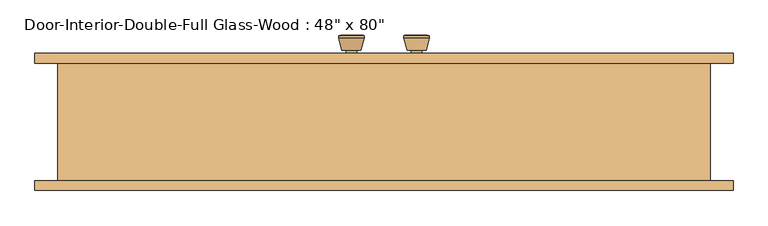
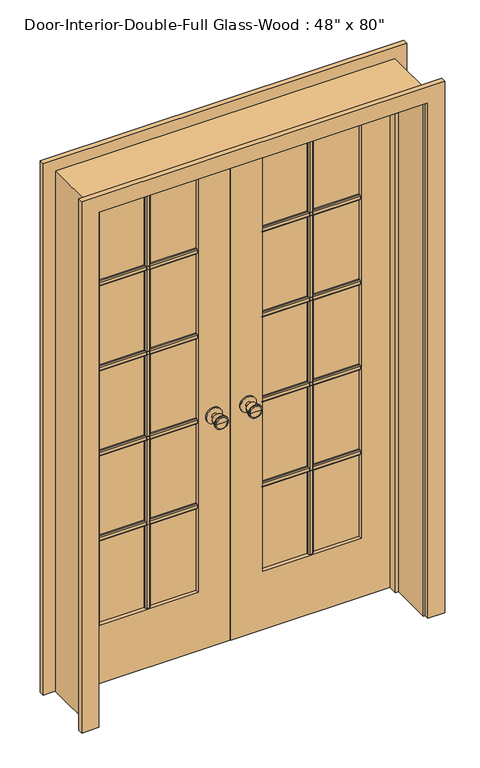
"""IFC4 building model written with IfcOpenShell, lengths in millimetres: door geometry."""

from ifc_helpers import new_model, si_unit, point, frame, frame_2d, origin, place, context, project, spatial, polyline, circle_curve, trimmed, segment, composite_curve, outline, extrude, faceted_brep, source, transform, mapped, element, save
from ifc_brep_helpers import plane_surface, cylinder_surface, revolved_surface, advanced_brep


def door_cd3c5da8(model_context):
    return source(origin(), model_context, "Body", "SolidModel", [
        advanced_brep(
        [(-63.5, 117.125, 914.4), (-73.5, 117.125, 914.4), (-53.5, 117.125, 914.4), (-83.9758676, 166.125, 914.4), (-63.5, 166.125, 914.4), (-43.0241324, 166.125, 914.4), (-88.5, 164.2971319, 914.4), (-38.5, 164.2971319, 914.4), (-88.5, 160.8334537, 914.4), (-38.5, 160.8334537, 914.4), (-82.136236, 136.125, 914.4), (-44.863764, 136.125, 914.4), (-73.5, 136.125, 914.4), (-53.5, 136.125, 914.4)],
        [
            (0, 1),
            (1, 2, circle_curve(frame((-63.5, 117.125, 914.4), z_axis=(0.0, -1.0, 0.0), x_axis=(1.0, 0.0, 0.0)), 10.0)),
            (2, 0),
            (2, 1, circle_curve(frame((-63.5, 117.125, 914.4), z_axis=(0.0, -1.0, 0.0), x_axis=(1.0, 0.0, 0.0)), 10.0)),
            (3, 4),
            (4, 5),
            (5, 3, circle_curve(frame((-63.5, 166.125, 914.4), z_axis=(0.0, 1.0, 0.0), x_axis=(1.0, 0.0, 0.0)), 20.4758676)),
            (3, 5, circle_curve(frame((-63.5, 166.125, 914.4), z_axis=(0.0, 1.0, 0.0), x_axis=(1.0, 0.0, 0.0)), 20.4758676)),
            (6, 3),
            (5, 7),
            (7, 6, circle_curve(frame((-63.5, 164.2971319, 914.4), z_axis=(0.0, 1.0, 0.0), x_axis=(1.0, 0.0, 0.0)), 25.0)),
            (6, 7, circle_curve(frame((-63.5, 164.2971319, 914.4), z_axis=(0.0, 1.0, 0.0), x_axis=(1.0, 0.0, 0.0)), 25.0)),
            (8, 6),
            (7, 9),
            (9, 8, circle_curve(frame((-63.5, 160.8334537, 914.4), z_axis=(0.0, 1.0, 0.0), x_axis=(1.0, 0.0, 0.0)), 25.0)),
            (8, 9, circle_curve(frame((-63.5, 160.8334537, 914.4), z_axis=(0.0, 1.0, 0.0), x_axis=(1.0, 0.0, 0.0)), 25.0)),
            (10, 8),
            (9, 11),
            (11, 10, circle_curve(frame((-63.5, 136.125, 914.4), z_axis=(0.0, 1.0, 0.0), x_axis=(1.0, 0.0, 0.0)), 18.636236)),
            (10, 11, circle_curve(frame((-63.5, 136.125, 914.4), z_axis=(0.0, 1.0, 0.0), x_axis=(1.0, 0.0, 0.0)), 18.636236)),
            (12, 10),
            (11, 13),
            (13, 12, circle_curve(frame((-63.5, 136.125, 914.4), z_axis=(0.0, 1.0, 0.0), x_axis=(1.0, 0.0, 0.0)), 10.0)),
            (12, 13, circle_curve(frame((-63.5, 136.125, 914.4), z_axis=(0.0, 1.0, 0.0), x_axis=(1.0, 0.0, 0.0)), 10.0)),
            (1, 12),
            (13, 2),
        ],
        [
            plane_surface(frame((-63.5, 117.125, 914.4), z_axis=(0.0, -1.0, 0.0), x_axis=(1.0, 0.0, 0.0))),
            plane_surface(frame((-63.5, 166.125, 914.4), z_axis=(0.0, 1.0, 0.0), x_axis=(1.0, 0.0, 0.0))),
            revolved_surface(polyline([(-43.0241324, 166.125, 914.4), (-38.5, 164.2971319, 914.4)]), (-63.5, 117.125, 914.4), (0.0, -1.0, 0.0)),
            cylinder_surface(frame((-63.5, 117.125, 914.4), z_axis=(0.0, -1.0, 0.0), x_axis=(1.0, 0.0, 0.0)), 25.0),
            revolved_surface(polyline([(-38.5, 160.8334537, 914.4), (-44.863764, 136.125, 914.4)]), (-63.5, 117.125, 914.4), (0.0, -1.0, 0.0)),
            plane_surface(frame((-63.5, 136.125, 914.4), z_axis=(0.0, -1.0, 0.0), x_axis=(1.0, 0.0, 0.0))),
            cylinder_surface(frame((-63.5, 117.125, 914.4), z_axis=(0.0, -1.0, 0.0), x_axis=(1.0, 0.0, 0.0)), 10.0),
        ],
        [
            (0, [[1, 2, 3]]),
            (0, [[-3, 4, -1]]),
            (1, [[5, 6, 7]]),
            (1, [[-6, -5, 8]]),
            (2, [[9, -7, 10, 11]]),
            (2, [[-10, -8, -9, 12]]),
            (3, [[13, -11, 14, 15]]),
            (3, [[-14, -12, -13, 16]]),
            (4, [[17, -15, 18, 19]]),
            (4, [[-18, -16, -17, 20]]),
            (5, [[21, -19, 22, 23]]),
            (5, [[-22, -20, -21, 24]]),
            (6, [[25, -23, 26, -2]]),
            (6, [[-26, -24, -25, -4]]),
        ],
    ),
        extrude(outline(composite_curve([segment(trimmed(circle_curve(frame_2d((914.4, -63.5)), 30.0), [point((914.4, -33.5))], [point((914.4, -93.5))], False, "CARTESIAN"), True, "CONTINUOUS"), segment(trimmed(circle_curve(frame_2d((914.4, -63.5)), 30.0), [point((914.4, -93.5))], [point((914.4, -33.5))], False, "CARTESIAN"), True, "CONTINUOUS")], self_intersect=False)), frame((0.0, 111.125, 0.0), z_axis=(0.0, 1.0, 0.0), x_axis=(0.0, 0.0, 1.0)), (0.0, 0.0, 1.0), 6.0),
        advanced_brep(
        [(-63.5, 70.2, 914.4), (-53.5, 70.2, 914.4), (-73.5, 70.2, 914.4), (-83.9758676, 21.2, 914.4), (-43.0241324, 21.2, 914.4), (-63.5, 21.2, 914.4), (-88.5, 23.0278681, 914.4), (-38.5, 23.0278681, 914.4), (-88.5, 26.4915463, 914.4), (-38.5, 26.4915463, 914.4), (-82.136236, 51.2, 914.4), (-44.863764, 51.2, 914.4), (-73.5, 51.2, 914.4), (-53.5, 51.2, 914.4)],
        [
            (0, 1),
            (1, 2, circle_curve(frame((-63.5, 70.2, 914.4), z_axis=(0.0, 1.0, 0.0), x_axis=(1.0, 0.0, 0.0)), 10.0)),
            (2, 0),
            (2, 1, circle_curve(frame((-63.5, 70.2, 914.4), z_axis=(0.0, 1.0, 0.0), x_axis=(1.0, 0.0, 0.0)), 10.0)),
            (3, 4, circle_curve(frame((-63.5, 21.2, 914.4), z_axis=(0.0, -1.0, 0.0), x_axis=(1.0, 0.0, 0.0)), 20.4758676)),
            (4, 5),
            (5, 3),
            (4, 3, circle_curve(frame((-63.5, 21.2, 914.4), z_axis=(0.0, -1.0, 0.0), x_axis=(1.0, 0.0, 0.0)), 20.4758676)),
            (6, 7, circle_curve(frame((-63.5, 23.0278681, 914.4), z_axis=(0.0, -1.0, 0.0), x_axis=(1.0, 0.0, 0.0)), 25.0)),
            (7, 4),
            (3, 6),
            (7, 6, circle_curve(frame((-63.5, 23.0278681, 914.4), z_axis=(0.0, -1.0, 0.0), x_axis=(1.0, 0.0, 0.0)), 25.0)),
            (8, 9, circle_curve(frame((-63.5, 26.4915463, 914.4), z_axis=(0.0, -1.0, 0.0), x_axis=(1.0, 0.0, 0.0)), 25.0)),
            (9, 7),
            (6, 8),
            (9, 8, circle_curve(frame((-63.5, 26.4915463, 914.4), z_axis=(0.0, -1.0, 0.0), x_axis=(1.0, 0.0, 0.0)), 25.0)),
            (10, 11, circle_curve(frame((-63.5, 51.2, 914.4), z_axis=(0.0, -1.0, 0.0), x_axis=(1.0, 0.0, 0.0)), 18.636236)),
            (11, 9),
            (8, 10),
            (11, 10, circle_curve(frame((-63.5, 51.2, 914.4), z_axis=(0.0, -1.0, 0.0), x_axis=(1.0, 0.0, 0.0)), 18.636236)),
            (12, 13, circle_curve(frame((-63.5, 51.2, 914.4), z_axis=(0.0, -1.0, 0.0), x_axis=(1.0, 0.0, 0.0)), 10.0)),
            (13, 11),
            (10, 12),
            (13, 12, circle_curve(frame((-63.5, 51.2, 914.4), z_axis=(0.0, -1.0, 0.0), x_axis=(1.0, 0.0, 0.0)), 10.0)),
            (1, 13),
            (12, 2),
        ],
        [
            plane_surface(frame((-63.5, 70.2, 914.4), z_axis=(0.0, 1.0, 0.0), x_axis=(1.0, 0.0, 0.0))),
            plane_surface(frame((-63.5, 21.2, 914.4), z_axis=(0.0, -1.0, 0.0), x_axis=(1.0, 0.0, 0.0))),
            revolved_surface(polyline([(-43.0241324, 21.2, 914.4), (-38.5, 23.0278681, 914.4)]), (-63.5, 70.2, 914.4), (0.0, 1.0, 0.0)),
            cylinder_surface(frame((-63.5, 70.2, 914.4), z_axis=(0.0, 1.0, 0.0), x_axis=(1.0, 0.0, 0.0)), 25.0),
            revolved_surface(polyline([(-38.5, 26.4915463, 914.4), (-44.863764, 51.2, 914.4)]), (-63.5, 70.2, 914.4), (0.0, 1.0, 0.0)),
            plane_surface(frame((-63.5, 51.2, 914.4), z_axis=(0.0, 1.0, 0.0), x_axis=(1.0, 0.0, 0.0))),
            cylinder_surface(frame((-63.5, 70.2, 914.4), z_axis=(0.0, 1.0, 0.0), x_axis=(1.0, 0.0, 0.0)), 10.0),
        ],
        [
            (0, [[1, 2, 3]]),
            (0, [[-3, 4, -1]]),
            (1, [[5, 6, 7]]),
            (1, [[8, -7, -6]]),
            (2, [[9, 10, -5, 11]]),
            (2, [[12, -11, -8, -10]]),
            (3, [[13, 14, -9, 15]]),
            (3, [[16, -15, -12, -14]]),
            (4, [[17, 18, -13, 19]]),
            (4, [[20, -19, -16, -18]]),
            (5, [[21, 22, -17, 23]]),
            (5, [[24, -23, -20, -22]]),
            (6, [[-2, 25, -21, 26]]),
            (6, [[-4, -26, -24, -25]]),
        ],
    ),
        extrude(outline(composite_curve([segment(trimmed(circle_curve(frame_2d((914.4, -63.5)), 30.0), [point((914.4, -33.5))], [point((914.4, -93.5))], False, "CARTESIAN"), True, "CONTINUOUS"), segment(trimmed(circle_curve(frame_2d((914.4, -63.5)), 30.0), [point((914.4, -93.5))], [point((914.4, -33.5))], False, "CARTESIAN"), True, "CONTINUOUS")], self_intersect=False)), frame((0.0, 70.2, 0.0), z_axis=(0.0, 1.0, 0.0), x_axis=(0.0, 0.0, 1.0)), (0.0, 0.0, 1.0), 6.0),
        extrude(outline(polyline([(90.17, 1586.23), (90.17, 1567.18), (83.82, 1567.18), (80.645, 1570.355), (80.645, 1583.055), (83.82, 1586.23), (90.17, 1586.23)])), frame((120.65, 0.0, 0.0), z_axis=(1.0, 0.0, 0.0), x_axis=(0.0, 1.0, 0.0)), (0.0, 0.0, 1.0), 368.3),
        extrude(outline(polyline([(90.17, 1249.9975), (90.17, 1230.9475), (83.82, 1230.9475), (80.645, 1234.1225), (80.645, 1246.8225), (83.82, 1249.9975), (90.17, 1249.9975)])), frame((120.65, 0.0, 0.0), z_axis=(1.0, 0.0, 0.0), x_axis=(0.0, 1.0, 0.0)), (0.0, 0.0, 1.0), 368.3),
        extrude(outline(polyline([(90.17, 913.765), (90.17, 894.715), (83.82, 894.715), (80.645, 897.89), (80.645, 910.59), (83.82, 913.765), (90.17, 913.765)])), frame((120.65, 0.0, 0.0), z_axis=(1.0, 0.0, 0.0), x_axis=(0.0, 1.0, 0.0)), (0.0, 0.0, 1.0), 368.3),
        extrude(outline(polyline([(295.275, 90.17), (314.325, 90.17), (314.325, 83.82), (311.15, 80.645), (298.45, 80.645), (295.275, 83.82), (295.275, 90.17)])), frame((0.0, 0.0, 231.775), z_axis=(0.0, 0.0, 1.0), x_axis=(1.0, 0.0, 0.0)), (0.0, 0.0, 1.0), 1681.1625),
        extrude(outline(polyline([(90.17, 577.5325), (90.17, 558.4825), (83.82, 558.4825), (80.645, 561.6575), (80.645, 574.3575), (83.82, 577.5325), (90.17, 577.5325)])), frame((120.65, 0.0, 0.0), z_axis=(1.0, 0.0, 0.0), x_axis=(0.0, 1.0, 0.0)), (0.0, 0.0, 1.0), 368.3),
        extrude(outline(polyline([(97.155, 1586.23), (103.505, 1586.23), (106.68, 1583.055), (106.68, 1570.355), (103.505, 1567.18), (97.155, 1567.18), (97.155, 1586.23)])), frame((-488.95, 0.0, 0.0), z_axis=(1.0, 0.0, 0.0), x_axis=(0.0, 1.0, 0.0)), (0.0, 0.0, 1.0), 368.3),
        extrude(outline(polyline([(97.155, 1249.9975), (103.505, 1249.9975), (106.68, 1246.8225), (106.68, 1234.1225), (103.505, 1230.9475), (97.155, 1230.9475), (97.155, 1249.9975)])), frame((-488.95, 0.0, 0.0), z_axis=(1.0, 0.0, 0.0), x_axis=(0.0, 1.0, 0.0)), (0.0, 0.0, 1.0), 368.3),
        extrude(outline(polyline([(97.155, 913.765), (103.505, 913.765), (106.68, 910.59), (106.68, 897.89), (103.505, 894.715), (97.155, 894.715), (97.155, 913.765)])), frame((-488.95, 0.0, 0.0), z_axis=(1.0, 0.0, 0.0), x_axis=(0.0, 1.0, 0.0)), (0.0, 0.0, 1.0), 368.3),
        extrude(outline(polyline([(-314.325, 97.155), (-314.325, 103.505), (-311.15, 106.68), (-298.45, 106.68), (-295.275, 103.505), (-295.275, 97.155), (-314.325, 97.155)])), frame((0.0, 0.0, 231.775), z_axis=(0.0, 0.0, 1.0), x_axis=(1.0, 0.0, 0.0)), (0.0, 0.0, 1.0), 1681.1625),
        extrude(outline(polyline([(97.155, 577.5325), (103.505, 577.5325), (106.68, 574.3575), (106.68, 561.6575), (103.505, 558.4825), (97.155, 558.4825), (97.155, 577.5325)])), frame((-488.95, 0.0, 0.0), z_axis=(1.0, 0.0, 0.0), x_axis=(0.0, 1.0, 0.0)), (0.0, 0.0, 1.0), 368.3),
        extrude(outline(polyline([(97.155, 1586.23), (103.505, 1586.23), (106.68, 1583.055), (106.68, 1570.355), (103.505, 1567.18), (97.155, 1567.18), (97.155, 1586.23)])), frame((120.65, 0.0, 0.0), z_axis=(1.0, 0.0, 0.0), x_axis=(0.0, 1.0, 0.0)), (0.0, 0.0, 1.0), 368.3),
        extrude(outline(polyline([(97.155, 1249.9975), (103.505, 1249.9975), (106.68, 1246.8225), (106.68, 1234.1225), (103.505, 1230.9475), (97.155, 1230.9475), (97.155, 1249.9975)])), frame((120.65, 0.0, 0.0), z_axis=(1.0, 0.0, 0.0), x_axis=(0.0, 1.0, 0.0)), (0.0, 0.0, 1.0), 368.3),
        extrude(outline(polyline([(97.155, 913.765), (103.505, 913.765), (106.68, 910.59), (106.68, 897.89), (103.505, 894.715), (97.155, 894.715), (97.155, 913.765)])), frame((120.65, 0.0, 0.0), z_axis=(1.0, 0.0, 0.0), x_axis=(0.0, 1.0, 0.0)), (0.0, 0.0, 1.0), 368.3),
        extrude(outline(polyline([(295.275, 97.155), (295.275, 103.505), (298.45, 106.68), (311.15, 106.68), (314.325, 103.505), (314.325, 97.155), (295.275, 97.155)])), frame((0.0, 0.0, 231.775), z_axis=(0.0, 0.0, 1.0), x_axis=(1.0, 0.0, 0.0)), (0.0, 0.0, 1.0), 1681.1625),
        extrude(outline(polyline([(97.155, 577.5325), (103.505, 577.5325), (106.68, 574.3575), (106.68, 561.6575), (103.505, 558.4825), (97.155, 558.4825), (97.155, 577.5325)])), frame((120.65, 0.0, 0.0), z_axis=(1.0, 0.0, 0.0), x_axis=(0.0, 1.0, 0.0)), (0.0, 0.0, 1.0), 368.3),
        extrude(outline(polyline([(90.17, 1586.23), (90.17, 1567.18), (83.82, 1567.18), (80.645, 1570.355), (80.645, 1583.055), (83.82, 1586.23), (90.17, 1586.23)])), frame((-488.95, 0.0, 0.0), z_axis=(1.0, 0.0, 0.0), x_axis=(0.0, 1.0, 0.0)), (0.0, 0.0, 1.0), 368.3),
        extrude(outline(polyline([(90.17, 1249.9975), (90.17, 1230.9475), (83.82, 1230.9475), (80.645, 1234.1225), (80.645, 1246.8225), (83.82, 1249.9975), (90.17, 1249.9975)])), frame((-488.95, 0.0, 0.0), z_axis=(1.0, 0.0, 0.0), x_axis=(0.0, 1.0, 0.0)), (0.0, 0.0, 1.0), 368.3),
        extrude(outline(polyline([(90.17, 913.765), (90.17, 894.715), (83.82, 894.715), (80.645, 897.89), (80.645, 910.59), (83.82, 913.765), (90.17, 913.765)])), frame((-488.95, 0.0, 0.0), z_axis=(1.0, 0.0, 0.0), x_axis=(0.0, 1.0, 0.0)), (0.0, 0.0, 1.0), 368.3),
        extrude(outline(polyline([(-314.325, 90.17), (-295.275, 90.17), (-295.275, 83.82), (-298.45, 80.645), (-311.15, 80.645), (-314.325, 83.82), (-314.325, 90.17)])), frame((0.0, 0.0, 231.775), z_axis=(0.0, 0.0, 1.0), x_axis=(1.0, 0.0, 0.0)), (0.0, 0.0, 1.0), 1681.1625),
        extrude(outline(polyline([(90.17, 577.5325), (90.17, 558.4825), (83.82, 558.4825), (80.645, 561.6575), (80.645, 574.3575), (83.82, 577.5325), (90.17, 577.5325)])), frame((-488.95, 0.0, 0.0), z_axis=(1.0, 0.0, 0.0), x_axis=(0.0, 1.0, 0.0)), (0.0, 0.0, 1.0), 368.3),
        advanced_brep(
        [(63.5, 70.2, 914.4), (73.5, 70.2, 914.4), (53.5, 70.2, 914.4), (83.9758676, 21.2, 914.4), (63.5, 21.2, 914.4), (43.0241324, 21.2, 914.4), (88.5, 23.0278681, 914.4), (38.5, 23.0278681, 914.4), (88.5, 26.4915463, 914.4), (38.5, 26.4915463, 914.4), (82.136236, 51.2, 914.4), (44.863764, 51.2, 914.4), (73.5, 51.2, 914.4), (53.5, 51.2, 914.4)],
        [
            (0, 1),
            (1, 2, circle_curve(frame((63.5, 70.2, 914.4), z_axis=(0.0, 1.0, 0.0), x_axis=(-1.0, 0.0, 0.0)), 10.0)),
            (2, 0),
            (2, 1, circle_curve(frame((63.5, 70.2, 914.4), z_axis=(0.0, 1.0, 0.0), x_axis=(-1.0, 0.0, 0.0)), 10.0)),
            (3, 4),
            (4, 5),
            (5, 3, circle_curve(frame((63.5, 21.2, 914.4), z_axis=(0.0, -1.0, 0.0), x_axis=(-1.0, 0.0, 0.0)), 20.4758676)),
            (3, 5, circle_curve(frame((63.5, 21.2, 914.4), z_axis=(0.0, -1.0, 0.0), x_axis=(-1.0, 0.0, 0.0)), 20.4758676)),
            (6, 3),
            (5, 7),
            (7, 6, circle_curve(frame((63.5, 23.0278681, 914.4), z_axis=(0.0, -1.0, 0.0), x_axis=(-1.0, 0.0, 0.0)), 25.0)),
            (6, 7, circle_curve(frame((63.5, 23.0278681, 914.4), z_axis=(0.0, -1.0, 0.0), x_axis=(-1.0, 0.0, 0.0)), 25.0)),
            (8, 6),
            (7, 9),
            (9, 8, circle_curve(frame((63.5, 26.4915463, 914.4), z_axis=(0.0, -1.0, 0.0), x_axis=(-1.0, 0.0, 0.0)), 25.0)),
            (8, 9, circle_curve(frame((63.5, 26.4915463, 914.4), z_axis=(0.0, -1.0, 0.0), x_axis=(-1.0, 0.0, 0.0)), 25.0)),
            (10, 8),
            (9, 11),
            (11, 10, circle_curve(frame((63.5, 51.2, 914.4), z_axis=(0.0, -1.0, 0.0), x_axis=(-1.0, 0.0, 0.0)), 18.636236)),
            (10, 11, circle_curve(frame((63.5, 51.2, 914.4), z_axis=(0.0, -1.0, 0.0), x_axis=(-1.0, 0.0, 0.0)), 18.636236)),
            (12, 10),
            (11, 13),
            (13, 12, circle_curve(frame((63.5, 51.2, 914.4), z_axis=(0.0, -1.0, 0.0), x_axis=(-1.0, 0.0, 0.0)), 10.0)),
            (12, 13, circle_curve(frame((63.5, 51.2, 914.4), z_axis=(0.0, -1.0, 0.0), x_axis=(-1.0, 0.0, 0.0)), 10.0)),
            (1, 12),
            (13, 2),
        ],
        [
            plane_surface(frame((63.5, 70.2, 914.4), z_axis=(0.0, 1.0, 0.0), x_axis=(-1.0, 0.0, 0.0))),
            plane_surface(frame((63.5, 21.2, 914.4), z_axis=(0.0, -1.0, 0.0), x_axis=(-1.0, 0.0, 0.0))),
            revolved_surface(polyline([(43.0241324, 21.2, 914.4), (38.5, 23.0278681, 914.4)]), (63.5, 70.2, 914.4), (0.0, 1.0, 0.0)),
            cylinder_surface(frame((63.5, 70.2, 914.4), z_axis=(0.0, 1.0, 0.0), x_axis=(-1.0, 0.0, 0.0)), 25.0),
            revolved_surface(polyline([(38.5, 26.4915463, 914.4), (44.863764, 51.2, 914.4)]), (63.5, 70.2, 914.4), (0.0, 1.0, 0.0)),
            plane_surface(frame((63.5, 51.2, 914.4), z_axis=(0.0, 1.0, 0.0), x_axis=(-1.0, 0.0, 0.0))),
            cylinder_surface(frame((63.5, 70.2, 914.4), z_axis=(0.0, 1.0, 0.0), x_axis=(-1.0, 0.0, 0.0)), 10.0),
        ],
        [
            (0, [[1, 2, 3]]),
            (0, [[-3, 4, -1]]),
            (1, [[5, 6, 7]]),
            (1, [[-6, -5, 8]]),
            (2, [[9, -7, 10, 11]]),
            (2, [[-10, -8, -9, 12]]),
            (3, [[13, -11, 14, 15]]),
            (3, [[-14, -12, -13, 16]]),
            (4, [[17, -15, 18, 19]]),
            (4, [[-18, -16, -17, 20]]),
            (5, [[21, -19, 22, 23]]),
            (5, [[-22, -20, -21, 24]]),
            (6, [[25, -23, 26, -2]]),
            (6, [[-26, -24, -25, -4]]),
        ],
    ),
        extrude(outline(composite_curve([segment(trimmed(circle_curve(frame_2d((914.4, 63.5)), 30.0), [point((914.4, 33.5))], [point((914.4, 93.5))], False, "CARTESIAN"), True, "CONTINUOUS"), segment(trimmed(circle_curve(frame_2d((914.4, 63.5)), 30.0), [point((914.4, 93.5))], [point((914.4, 33.5))], False, "CARTESIAN"), True, "CONTINUOUS")], self_intersect=False)), frame((0.0, 70.2, 0.0), z_axis=(0.0, 1.0, 0.0), x_axis=(0.0, 0.0, 1.0)), (0.0, 0.0, 1.0), 6.0),
        advanced_brep(
        [(63.5, 117.125, 914.4), (53.5, 117.125, 914.4), (73.5, 117.125, 914.4), (83.9758676, 166.125, 914.4), (43.0241324, 166.125, 914.4), (63.5, 166.125, 914.4), (88.5, 164.2971319, 914.4), (38.5, 164.2971319, 914.4), (88.5, 160.8334537, 914.4), (38.5, 160.8334537, 914.4), (82.136236, 136.125, 914.4), (44.863764, 136.125, 914.4), (73.5, 136.125, 914.4), (53.5, 136.125, 914.4)],
        [
            (0, 1),
            (1, 2, circle_curve(frame((63.5, 117.125, 914.4), z_axis=(0.0, -1.0, 0.0), x_axis=(-1.0, 0.0, 0.0)), 10.0)),
            (2, 0),
            (2, 1, circle_curve(frame((63.5, 117.125, 914.4), z_axis=(0.0, -1.0, 0.0), x_axis=(-1.0, 0.0, 0.0)), 10.0)),
            (3, 4, circle_curve(frame((63.5, 166.125, 914.4), z_axis=(0.0, 1.0, 0.0), x_axis=(-1.0, 0.0, 0.0)), 20.4758676)),
            (4, 5),
            (5, 3),
            (4, 3, circle_curve(frame((63.5, 166.125, 914.4), z_axis=(0.0, 1.0, 0.0), x_axis=(-1.0, 0.0, 0.0)), 20.4758676)),
            (6, 7, circle_curve(frame((63.5, 164.2971319, 914.4), z_axis=(0.0, 1.0, 0.0), x_axis=(-1.0, 0.0, 0.0)), 25.0)),
            (7, 4),
            (3, 6),
            (7, 6, circle_curve(frame((63.5, 164.2971319, 914.4), z_axis=(0.0, 1.0, 0.0), x_axis=(-1.0, 0.0, 0.0)), 25.0)),
            (8, 9, circle_curve(frame((63.5, 160.8334537, 914.4), z_axis=(0.0, 1.0, 0.0), x_axis=(-1.0, 0.0, 0.0)), 25.0)),
            (9, 7),
            (6, 8),
            (9, 8, circle_curve(frame((63.5, 160.8334537, 914.4), z_axis=(0.0, 1.0, 0.0), x_axis=(-1.0, 0.0, 0.0)), 25.0)),
            (10, 11, circle_curve(frame((63.5, 136.125, 914.4), z_axis=(0.0, 1.0, 0.0), x_axis=(-1.0, 0.0, 0.0)), 18.636236)),
            (11, 9),
            (8, 10),
            (11, 10, circle_curve(frame((63.5, 136.125, 914.4), z_axis=(0.0, 1.0, 0.0), x_axis=(-1.0, 0.0, 0.0)), 18.636236)),
            (12, 13, circle_curve(frame((63.5, 136.125, 914.4), z_axis=(0.0, 1.0, 0.0), x_axis=(-1.0, 0.0, 0.0)), 10.0)),
            (13, 11),
            (10, 12),
            (13, 12, circle_curve(frame((63.5, 136.125, 914.4), z_axis=(0.0, 1.0, 0.0), x_axis=(-1.0, 0.0, 0.0)), 10.0)),
            (1, 13),
            (12, 2),
        ],
        [
            plane_surface(frame((63.5, 117.125, 914.4), z_axis=(0.0, -1.0, 0.0), x_axis=(-1.0, 0.0, 0.0))),
            plane_surface(frame((63.5, 166.125, 914.4), z_axis=(0.0, 1.0, 0.0), x_axis=(-1.0, 0.0, 0.0))),
            revolved_surface(polyline([(43.0241324, 166.125, 914.4), (38.5, 164.2971319, 914.4)]), (63.5, 117.125, 914.4), (0.0, -1.0, 0.0)),
            cylinder_surface(frame((63.5, 117.125, 914.4), z_axis=(0.0, -1.0, 0.0), x_axis=(-1.0, 0.0, 0.0)), 25.0),
            revolved_surface(polyline([(38.5, 160.8334537, 914.4), (44.863764, 136.125, 914.4)]), (63.5, 117.125, 914.4), (0.0, -1.0, 0.0)),
            plane_surface(frame((63.5, 136.125, 914.4), z_axis=(0.0, -1.0, 0.0), x_axis=(-1.0, 0.0, 0.0))),
            cylinder_surface(frame((63.5, 117.125, 914.4), z_axis=(0.0, -1.0, 0.0), x_axis=(-1.0, 0.0, 0.0)), 10.0),
        ],
        [
            (0, [[1, 2, 3]]),
            (0, [[-3, 4, -1]]),
            (1, [[5, 6, 7]]),
            (1, [[8, -7, -6]]),
            (2, [[9, 10, -5, 11]]),
            (2, [[12, -11, -8, -10]]),
            (3, [[13, 14, -9, 15]]),
            (3, [[16, -15, -12, -14]]),
            (4, [[17, 18, -13, 19]]),
            (4, [[20, -19, -16, -18]]),
            (5, [[21, 22, -17, 23]]),
            (5, [[24, -23, -20, -22]]),
            (6, [[-2, 25, -21, 26]]),
            (6, [[-4, -26, -24, -25]]),
        ],
    ),
        extrude(outline(composite_curve([segment(trimmed(circle_curve(frame_2d((914.4, 63.5)), 30.0), [point((914.4, 33.5))], [point((914.4, 93.5))], False, "CARTESIAN"), True, "CONTINUOUS"), segment(trimmed(circle_curve(frame_2d((914.4, 63.5)), 30.0), [point((914.4, 93.5))], [point((914.4, 33.5))], False, "CARTESIAN"), True, "CONTINUOUS")], self_intersect=False)), frame((0.0, 111.125, 0.0), z_axis=(0.0, 1.0, 0.0), x_axis=(0.0, 0.0, 1.0)), (0.0, 0.0, 1.0), 6.0),
        extrude(outline(polyline([(0.0, 615.95), (0.0, 679.45), (2101.85, 679.45), (2101.85, -679.45), (0.0, -679.45), (0.0, -615.95), (2038.35, -615.95), (2038.35, 615.95), (0.0, 615.95)])), frame((0.0, -136.525, 0.0), z_axis=(0.0, 1.0, 0.0), x_axis=(0.0, 0.0, 1.0)), (0.0, 0.0, 1.0), 19.05),
        extrude(outline(polyline([(0.0, 615.95), (0.0, 679.45), (2101.85, 679.45), (2101.85, -679.45), (0.0, -679.45), (0.0, -615.95), (2038.35, -615.95), (2038.35, 615.95), (0.0, 615.95)])), frame((0.0, 111.125, 0.0), z_axis=(0.0, 1.0, 0.0), x_axis=(0.0, 0.0, 1.0)), (0.0, 0.0, 1.0), 19.05),
        faceted_brep([(635.0, 111.125, 0.0), (635.0, -117.475, 0.0), (609.6, -117.475, 0.0), (609.6, 41.275, 0.0), (596.9, 41.275, 0.0), (596.9, 76.2, 0.0), (609.6, 76.2, 0.0), (609.6, 111.125, 0.0), (635.0, 111.125, 2057.4), (635.0, -117.475, 2057.4), (-635.0, -117.475, 2057.4), (-635.0, -117.475, 0.0), (-609.6, -117.475, 0.0), (-609.6, -117.475, 2032.0), (609.6, -117.475, 2032.0), (609.6, 41.275, 2032.0), (-609.6, 41.275, 2032.0), (-609.6, 41.275, 0.0), (-596.9, 41.275, 0.0), (-596.9, 41.275, 2019.3), (596.9, 41.275, 2019.3), (596.9, 76.2, 2019.3), (1.5875, 76.2, 2019.3), (-1.6019111, 76.2, 2019.3), (-596.9, 76.2, 2019.3), (-596.9, 76.2, 0.0), (-609.6, 76.2, 0.0), (-609.6, 76.2, 2032.0), (-1.6019111, 76.2, 2032.0), (1.5875, 76.2, 2032.0), (609.6, 76.2, 2032.0), (609.6, 111.125, 2032.0), (1.5875, 111.125, 2032.0), (-1.6019111, 111.125, 2032.0), (-609.6, 111.125, 2032.0), (-609.6, 111.125, 0.0), (-635.0, 111.125, 0.0), (-635.0, 111.125, 2057.4)], [[[0, 1, 2, 3, 4, 5, 6, 7]], [[1, 0, 8, 9]], [[2, 1, 9, 10, 11, 12, 13, 14]], [[3, 2, 14, 15]], [[4, 3, 15, 16, 17, 18, 19, 20]], [[5, 4, 20, 21]], [[6, 5, 21, 22, 23, 24, 25, 26, 27, 28, 29, 30]], [[7, 6, 30, 31]], [[0, 7, 31, 32, 33, 34, 35, 36, 37, 8]], [[9, 8, 37, 10]], [[14, 13, 16, 15]], [[20, 19, 24, 23, 22, 21]], [[31, 30, 29, 28, 27, 34, 33, 32]], [[12, 11, 36, 35, 26, 25, 18, 17]], [[11, 10, 37, 36]], [[13, 12, 17, 16]], [[19, 18, 25, 24]], [[27, 26, 35, 34]]]),
        extrude(outline(polyline([(2032.0, -609.6), (0.0, -609.6), (0.0, -1.6019111), (2032.0, -1.6019111), (2032.0, -609.6)]), holes=[polyline([(231.775, -488.95), (1912.9375, -488.95), (1912.9375, -120.65), (231.775, -120.65), (231.775, -488.95)])]), frame((0.0, 76.2, 0.0), z_axis=(0.0, 1.0, 0.0), x_axis=(0.0, 0.0, 1.0)), (0.0, 0.0, 1.0), 34.925),
        extrude(outline(polyline([(0.0, 609.6), (2032.0, 609.6), (2032.0, 1.5875), (0.0, 1.5875), (0.0, 609.6)]), holes=[polyline([(1912.9375, 120.65), (1912.9375, 488.95), (231.775, 488.95), (231.775, 120.65), (1912.9375, 120.65)])]), frame((0.0, 76.2, 0.0), z_axis=(0.0, 1.0, 0.0), x_axis=(0.0, 0.0, 1.0)), (0.0, 0.0, 1.0), 34.925),
        extrude(outline(polyline([(488.95, 90.17), (120.65, 90.17), (120.65, 97.155), (488.95, 97.155), (488.95, 90.17)])), frame((0.0, 0.0, 231.775), z_axis=(0.0, 0.0, 1.0), x_axis=(1.0, 0.0, 0.0)), (0.0, 0.0, 1.0), 1681.1625),
        extrude(outline(polyline([(-120.65, 90.17), (-488.95, 90.17), (-488.95, 97.155), (-120.65, 97.155), (-120.65, 90.17)])), frame((0.0, 0.0, 231.775), z_axis=(0.0, 0.0, 1.0), x_axis=(1.0, 0.0, 0.0)), (0.0, 0.0, 1.0), 1681.1625),
    ])


if __name__ == "__main__":
    model = new_model("IFC4")
    model_context = context("Model", 3, world=origin())
    ifc_project = project(units=[si_unit("LENGTHUNIT", "METRE", prefix="MILLI")], contexts=[model_context])
    site = spatial("IfcSite", under=ifc_project)
    building = spatial("IfcBuilding", under=site)
    placement = place(None, origin())
    door_shape = door_cd3c5da8(model_context)
    element("IfcDoor", 1, ObjectType="Door-Interior-Double-Full Glass-Wood : 48\" x 80\"", at=placement, inside=building, context=model_context, shape_type="MappedRepresentation", body=[
        mapped(door_shape, transform((0.0, 0.0, 0.0), x_axis=(1.0, 0.0, 0.0), y_axis=(0.0, 1.0, 0.0), z_axis=(0.0, 0.0, 1.0))),
    ])
    save(model, "model.ifc")

# Revit data of these elements
# Type "Door-Interior-Double-Full Glass-Wood : 48\" x 80\""
#   Type Mark = "11"
#   Assembly Code = "C1020300"
#   Analytic Construction = "French door, wood frame with single glass"
#   Top Rail = 0' - 4 11/16"
#   Thickness = 0' - 1 3/8"
#   Thermal Resistance (R) = 1.0696 (h·ft²·°F)/BTU
#   Swing Angle [instance default] = 90.00°
#   Stiles = 0' - 4 3/4"
#   Rough Width = 4' - 2"
#   Rough Height = 6' - 9"
#   Panel Width = 2' - 0"
#   Height = 6' - 8"
#   Width = 4' - 0"
#   Heat Transfer Coefficient (U) = 0.9350 BTU/(h·ft²·°F)
#   Bottom Rail = 0' - 9 1/8"
#   Show Grill [instance default] = yes
#   Trim Material = Cherry
#   Panel Material = Cherry
#   Frame Material = Cherry
#   Door Handle Material = Aluminum
#   Visual Light Transmittance = 0
#   Solar Heat Gain Coefficient = 0
#   Wall Closure = (empty or 0)
#   Function = (empty or 0)
# Element 1 (IfcDoor, "Door-Interior-Double-Full Glass-Wood : 48\" x 80\"")
#   Materials on its faces: "Cherry", "Aluminum", "Glass"
# Materials
#   "Cherry": class "Wood", colour RGB 226 177 128, transparency 0, Description = "Prunus Serotina", Cost = 0
#   "Aluminum": class "Metal", colour RGB 247 247 247, transparency 0, Description = "Aluminum 6061", Cost = 0
#   "Glass": class "Glass", colour RGB 0 128 192, transparency 0.75, Description = "Soda Lime Glass", Cost = 0
